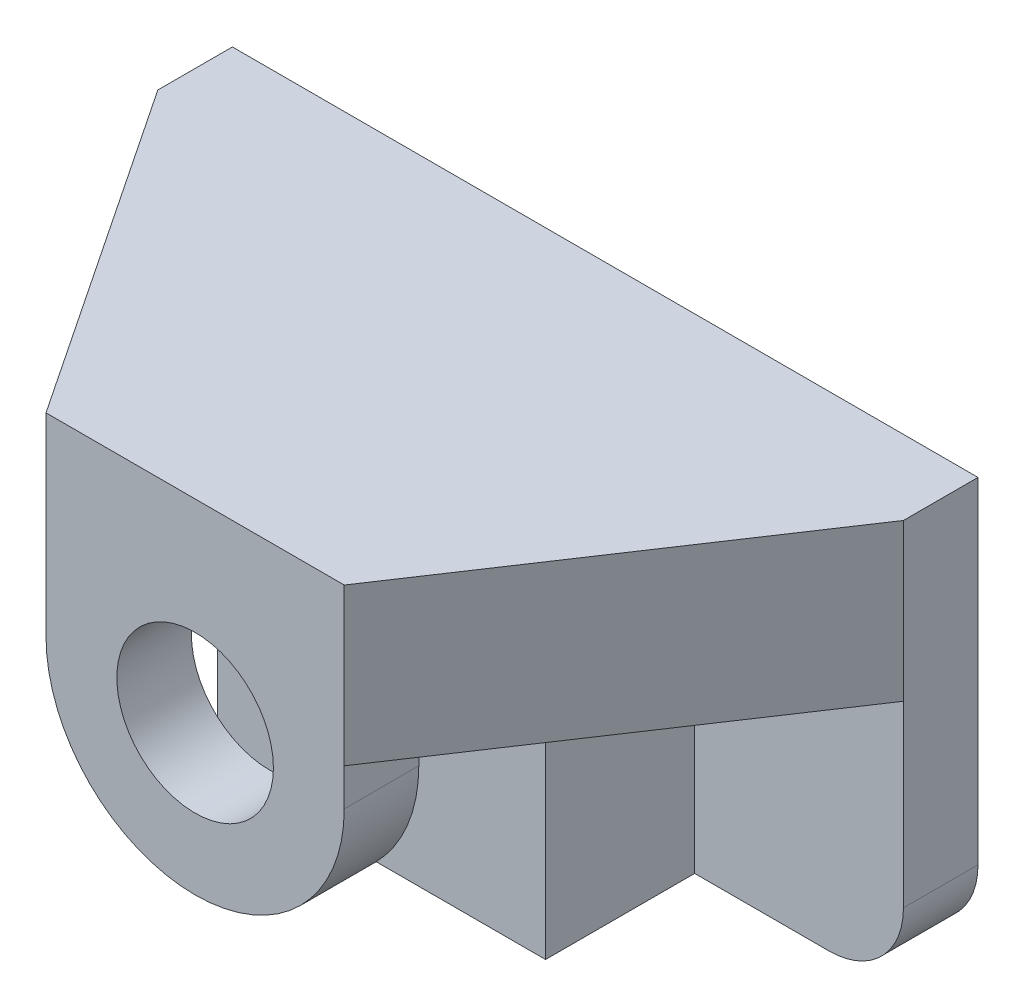
ISO-10303-21;
HEADER;
FILE_DESCRIPTION(('STEP AP214'),'2;1');
FILE_NAME('part.step','',(''),(''),'','','');
FILE_SCHEMA(('AUTOMOTIVE_DESIGN { 1 0 10303 214 1 1 1 1 }'));
ENDSEC;
DATA;
#1=APPLICATION_CONTEXT('core data for automotive mechanical design processes');
#2=APPLICATION_PROTOCOL_DEFINITION('international standard','automotive_design',2000,#1);
#3=PRODUCT_CONTEXT('',#1,'mechanical');
#4=PRODUCT('Part','Part','',(#3));
#5=PRODUCT_RELATED_PRODUCT_CATEGORY('part','',(#4));
#6=PRODUCT_DEFINITION_FORMATION('','',#4);
#7=PRODUCT_DEFINITION_CONTEXT('part definition',#1,'design');
#8=PRODUCT_DEFINITION('design','',#6,#7);
#9=PRODUCT_DEFINITION_SHAPE('','',#8);
#10=(LENGTH_UNIT() NAMED_UNIT(*) SI_UNIT(.MILLI.,.METRE.));
#11=(NAMED_UNIT(*) PLANE_ANGLE_UNIT() SI_UNIT($,.RADIAN.));
#12=(NAMED_UNIT(*) SI_UNIT($,.STERADIAN.) SOLID_ANGLE_UNIT());
#13=UNCERTAINTY_MEASURE_WITH_UNIT(LENGTH_MEASURE(1.E-05),#10,'distance_accuracy_value','');
#14=(GEOMETRIC_REPRESENTATION_CONTEXT(3) GLOBAL_UNCERTAINTY_ASSIGNED_CONTEXT((#13)) GLOBAL_UNIT_ASSIGNED_CONTEXT((#10,
#11,#12)) REPRESENTATION_CONTEXT('',''));
#15=CARTESIAN_POINT('',(0.,0.,0.));
#16=DIRECTION('',(0.,0.,1.));
#17=DIRECTION('',(1.,0.,0.));
#18=AXIS2_PLACEMENT_3D('',#15,#16,#17);
#19=CARTESIAN_POINT('',(0.,-21.,0.));
#20=DIRECTION('',(0.,-1.,0.));
#21=DIRECTION('',(0.,0.,-1.));
#22=AXIS2_PLACEMENT_3D('',#19,#20,#21);
#23=PLANE('',#22);
#24=DIRECTION('',(1.,0.,0.));
#25=VECTOR('',#24,1.);
#26=CARTESIAN_POINT('',(20.,-21.,45.));
#27=LINE('',#26,#25);
#28=CARTESIAN_POINT('',(-20.,-21.,45.));
#29=VERTEX_POINT('',#28);
#30=CARTESIAN_POINT('',(-9.23309265630969,-21.,45.));
#31=VERTEX_POINT('',#30);
#32=EDGE_CURVE('E188',#29,#31,#27,.T.);
#33=ORIENTED_EDGE('',*,*,#32,.F.);
#34=DIRECTION('',(0.,0.,-1.));
#35=VECTOR('',#34,1.);
#36=CARTESIAN_POINT('',(-20.,-21.,45.));
#37=LINE('',#36,#35);
#38=CARTESIAN_POINT('',(-20.,-21.,55.));
#39=VERTEX_POINT('',#38);
#40=EDGE_CURVE('E205',#39,#29,#37,.T.);
#41=ORIENTED_EDGE('',*,*,#40,.F.);
#42=DIRECTION('',(0.554700196225229,0.,0.832050294337844));
#43=VECTOR('',#42,1.);
#44=CARTESIAN_POINT('',(-20.,-21.,55.));
#45=LINE('',#44,#43);
#46=CARTESIAN_POINT('',(-50.,-21.,10.));
#47=VERTEX_POINT('',#46);
#48=EDGE_CURVE('E247',#47,#39,#45,.T.);
#49=ORIENTED_EDGE('',*,*,#48,.F.);
#50=DIRECTION('',(-1.,0.,0.));
#51=VECTOR('',#50,1.);
#52=CARTESIAN_POINT('',(50.,-21.,10.));
#53=LINE('',#52,#51);
#54=CARTESIAN_POINT('',(-22.,-21.,10.));
#55=VERTEX_POINT('',#54);
#56=EDGE_CURVE('E259',#55,#47,#53,.T.);
#57=ORIENTED_EDGE('',*,*,#56,.F.);
#58=DIRECTION('',(0.,0.,1.));
#59=VECTOR('',#58,1.);
#60=CARTESIAN_POINT('',(-22.,-21.,30.));
#61=LINE('',#60,#59);
#62=CARTESIAN_POINT('',(-22.,-21.,30.));
#63=VERTEX_POINT('',#62);
#64=EDGE_CURVE('E267',#55,#63,#61,.T.);
#65=ORIENTED_EDGE('',*,*,#64,.T.);
#66=DIRECTION('',(1.,0.,0.));
#67=VECTOR('',#66,1.);
#68=CARTESIAN_POINT('',(22.0000000000001,-21.,30.));
#69=LINE('',#68,#67);
#70=CARTESIAN_POINT('',(22.0000000000001,-21.,30.));
#71=VERTEX_POINT('',#70);
#72=EDGE_CURVE('E273',#63,#71,#69,.T.);
#73=ORIENTED_EDGE('',*,*,#72,.T.);
#74=DIRECTION('',(0.,0.,-1.));
#75=VECTOR('',#74,1.);
#76=CARTESIAN_POINT('',(22.0000000000001,-21.,10.));
#77=LINE('',#76,#75);
#78=CARTESIAN_POINT('',(22.0000000000001,-21.,10.));
#79=VERTEX_POINT('',#78);
#80=EDGE_CURVE('E279',#71,#79,#77,.T.);
#81=ORIENTED_EDGE('',*,*,#80,.T.);
#82=CARTESIAN_POINT('',(50.,-21.,10.));
#83=VERTEX_POINT('',#82);
#84=EDGE_CURVE('E371',#83,#79,#53,.T.);
#85=ORIENTED_EDGE('',*,*,#84,.F.);
#86=DIRECTION('',(0.554700196225229,0.,-0.832050294337844));
#87=VECTOR('',#86,1.);
#88=CARTESIAN_POINT('',(20.,-21.,55.));
#89=LINE('',#88,#87);
#90=CARTESIAN_POINT('',(20.,-21.,55.));
#91=VERTEX_POINT('',#90);
#92=EDGE_CURVE('E253',#91,#83,#89,.T.);
#93=ORIENTED_EDGE('',*,*,#92,.F.);
#94=DIRECTION('',(0.,0.,1.));
#95=VECTOR('',#94,1.);
#96=CARTESIAN_POINT('',(20.,-21.,55.));
#97=LINE('',#96,#95);
#98=CARTESIAN_POINT('',(20.,-21.,45.));
#99=VERTEX_POINT('',#98);
#100=EDGE_CURVE('E196',#99,#91,#97,.T.);
#101=ORIENTED_EDGE('',*,*,#100,.F.);
#102=CARTESIAN_POINT('',(9.23309265630969,-21.,45.));
#103=VERTEX_POINT('',#102);
#104=EDGE_CURVE('E195',#103,#99,#27,.T.);
#105=ORIENTED_EDGE('',*,*,#104,.F.);
#106=EDGE_CURVE('E182',#31,#103,#27,.T.);
#107=ORIENTED_EDGE('',*,*,#106,.F.);
#108=EDGE_LOOP('',(#33,#41,#49,#57,#65,#73,#81,#85,#93,#101,#105,#107));
#109=FACE_BOUND('',#108,.T.);
#110=ADVANCED_FACE('F50',(#109),#23,.T.);
#111=CARTESIAN_POINT('',(0.,0.,10.));
#112=DIRECTION('',(0.,0.,1.));
#113=DIRECTION('',(1.,0.,0.));
#114=AXIS2_PLACEMENT_3D('',#111,#112,#113);
#115=PLANE('',#114);
#116=ORIENTED_EDGE('',*,*,#56,.T.);
#117=DIRECTION('',(0.,-1.,0.));
#118=VECTOR('',#117,1.);
#119=CARTESIAN_POINT('',(-50.,0.,10.));
#120=LINE('',#119,#118);
#121=CARTESIAN_POINT('',(-50.,-45.,10.));
#122=VERTEX_POINT('',#121);
#123=EDGE_CURVE('E303',#47,#122,#120,.T.);
#124=ORIENTED_EDGE('',*,*,#123,.T.);
#125=CARTESIAN_POINT('',(-40.,-45.,10.));
#126=DIRECTION('',(0.,0.,1.));
#127=DIRECTION('',(1.,0.,0.));
#128=AXIS2_PLACEMENT_3D('',#125,#126,#127);
#129=CIRCLE('',#128,9.99999999999999);
#130=CARTESIAN_POINT('',(-40.,-55.,10.));
#131=VERTEX_POINT('',#130);
#132=EDGE_CURVE('E306',#122,#131,#129,.T.);
#133=ORIENTED_EDGE('',*,*,#132,.T.);
#134=DIRECTION('',(1.,0.,0.));
#135=VECTOR('',#134,1.);
#136=CARTESIAN_POINT('',(0.,-55.,10.));
#137=LINE('',#136,#135);
#138=CARTESIAN_POINT('',(-22.,-55.,10.));
#139=VERTEX_POINT('',#138);
#140=EDGE_CURVE('E308',#131,#139,#137,.T.);
#141=ORIENTED_EDGE('',*,*,#140,.T.);
#142=DIRECTION('',(0.,1.,0.));
#143=VECTOR('',#142,1.);
#144=CARTESIAN_POINT('',(-22.,0.,10.));
#145=LINE('',#144,#143);
#146=EDGE_CURVE('E311',#139,#55,#145,.T.);
#147=ORIENTED_EDGE('',*,*,#146,.T.);
#148=EDGE_LOOP('',(#116,#124,#133,#141,#147));
#149=FACE_BOUND('',#148,.T.);
#150=ADVANCED_FACE('F415',(#149),#115,.T.);
#151=ORIENTED_EDGE('',*,*,#84,.T.);
#152=DIRECTION('',(0.,1.,0.));
#153=VECTOR('',#152,1.);
#154=CARTESIAN_POINT('',(22.0000000000001,0.,10.));
#155=LINE('',#154,#153);
#156=CARTESIAN_POINT('',(22.0000000000001,-55.,10.));
#157=VERTEX_POINT('',#156);
#158=EDGE_CURVE('E312',#157,#79,#155,.T.);
#159=ORIENTED_EDGE('',*,*,#158,.F.);
#160=DIRECTION('',(-1.,0.,0.));
#161=VECTOR('',#160,1.);
#162=CARTESIAN_POINT('',(0.,-55.,10.));
#163=LINE('',#162,#161);
#164=CARTESIAN_POINT('',(40.0000000000001,-55.,10.));
#165=VERTEX_POINT('',#164);
#166=EDGE_CURVE('E294',#165,#157,#163,.T.);
#167=ORIENTED_EDGE('',*,*,#166,.F.);
#168=CARTESIAN_POINT('',(40.,-45.,10.));
#169=DIRECTION('',(0.,0.,1.));
#170=DIRECTION('',(1.,0.,0.));
#171=AXIS2_PLACEMENT_3D('',#168,#169,#170);
#172=CIRCLE('',#171,10.);
#173=CARTESIAN_POINT('',(50.,-45.,10.));
#174=VERTEX_POINT('',#173);
#175=EDGE_CURVE('E296',#165,#174,#172,.T.);
#176=ORIENTED_EDGE('',*,*,#175,.T.);
#177=DIRECTION('',(0.,-1.,0.));
#178=VECTOR('',#177,1.);
#179=CARTESIAN_POINT('',(50.,0.,10.));
#180=LINE('',#179,#178);
#181=EDGE_CURVE('E69',#83,#174,#180,.T.);
#182=ORIENTED_EDGE('',*,*,#181,.F.);
#183=EDGE_LOOP('',(#151,#159,#167,#176,#182));
#184=FACE_BOUND('',#183,.T.);
#185=ADVANCED_FACE('F395',(#184),#115,.T.);
#186=CARTESIAN_POINT('',(40.,-45.,10.));
#187=DIRECTION('',(0.,0.,-1.));
#188=DIRECTION('',(-1.,0.,0.));
#189=AXIS2_PLACEMENT_3D('',#186,#187,#188);
#190=CYLINDRICAL_SURFACE('',#189,10.);
#191=CARTESIAN_POINT('',(40.,-45.,0.));
#192=DIRECTION('',(0.,0.,1.));
#193=DIRECTION('',(1.,0.,0.));
#194=AXIS2_PLACEMENT_3D('',#191,#192,#193);
#195=CIRCLE('',#194,10.);
#196=CARTESIAN_POINT('',(40.0000000000001,-55.,0.));
#197=VERTEX_POINT('',#196);
#198=CARTESIAN_POINT('',(50.,-45.,0.));
#199=VERTEX_POINT('',#198);
#200=EDGE_CURVE('E295',#197,#199,#195,.T.);
#201=ORIENTED_EDGE('',*,*,#200,.T.);
#202=DIRECTION('',(0.,0.,-1.));
#203=VECTOR('',#202,1.);
#204=CARTESIAN_POINT('',(50.,-45.,10.));
#205=LINE('',#204,#203);
#206=EDGE_CURVE('E338',#174,#199,#205,.T.);
#207=ORIENTED_EDGE('',*,*,#206,.F.);
#208=ORIENTED_EDGE('',*,*,#175,.F.);
#209=DIRECTION('',(0.,0.,-1.));
#210=VECTOR('',#209,1.);
#211=CARTESIAN_POINT('',(40.0000000000001,-55.,10.));
#212=LINE('',#211,#210);
#213=EDGE_CURVE('E345',#165,#197,#212,.T.);
#214=ORIENTED_EDGE('',*,*,#213,.T.);
#215=EDGE_LOOP('',(#201,#207,#208,#214));
#216=FACE_BOUND('',#215,.T.);
#217=ADVANCED_FACE('F47',(#216),#190,.T.);
#218=CARTESIAN_POINT('',(50.,0.,10.));
#219=DIRECTION('',(1.,0.,0.));
#220=DIRECTION('',(0.,0.,-1.));
#221=AXIS2_PLACEMENT_3D('',#218,#219,#220);
#222=PLANE('',#221);
#223=DIRECTION('',(0.,-1.,0.));
#224=VECTOR('',#223,1.);
#225=CARTESIAN_POINT('',(50.,0.,0.));
#226=LINE('',#225,#224);
#227=CARTESIAN_POINT('',(50.,0.,0.));
#228=VERTEX_POINT('',#227);
#229=EDGE_CURVE('E316',#228,#199,#226,.T.);
#230=ORIENTED_EDGE('',*,*,#229,.F.);
#231=DIRECTION('',(0.,0.,-1.));
#232=VECTOR('',#231,1.);
#233=CARTESIAN_POINT('',(50.,0.,10.));
#234=LINE('',#233,#232);
#235=CARTESIAN_POINT('',(50.,0.,10.));
#236=VERTEX_POINT('',#235);
#237=EDGE_CURVE('E336',#236,#228,#234,.T.);
#238=ORIENTED_EDGE('',*,*,#237,.F.);
#239=EDGE_CURVE('E301',#236,#83,#180,.T.);
#240=ORIENTED_EDGE('',*,*,#239,.T.);
#241=ORIENTED_EDGE('',*,*,#181,.T.);
#242=ORIENTED_EDGE('',*,*,#206,.T.);
#243=EDGE_LOOP('',(#230,#238,#240,#241,#242));
#244=FACE_BOUND('',#243,.T.);
#245=ADVANCED_FACE('F401',(#244),#222,.T.);
#246=CARTESIAN_POINT('',(0.,0.,10.));
#247=DIRECTION('',(0.,1.,0.));
#248=DIRECTION('',(0.,0.,1.));
#249=AXIS2_PLACEMENT_3D('',#246,#247,#248);
#250=PLANE('',#249);
#251=DIRECTION('',(1.,0.,0.));
#252=VECTOR('',#251,1.);
#253=CARTESIAN_POINT('',(0.,0.,0.));
#254=LINE('',#253,#252);
#255=CARTESIAN_POINT('',(-50.,0.,0.));
#256=VERTEX_POINT('',#255);
#257=EDGE_CURVE('E325',#256,#228,#254,.T.);
#258=ORIENTED_EDGE('',*,*,#257,.F.);
#259=DIRECTION('',(0.,0.,-1.));
#260=VECTOR('',#259,1.);
#261=CARTESIAN_POINT('',(-50.,0.,10.));
#262=LINE('',#261,#260);
#263=CARTESIAN_POINT('',(-50.,0.,10.));
#264=VERTEX_POINT('',#263);
#265=EDGE_CURVE('E254',#264,#256,#262,.T.);
#266=ORIENTED_EDGE('',*,*,#265,.F.);
#267=DIRECTION('',(0.554700196225229,0.,0.832050294337844));
#268=VECTOR('',#267,1.);
#269=CARTESIAN_POINT('',(-20.,0.,55.));
#270=LINE('',#269,#268);
#271=CARTESIAN_POINT('',(-20.,0.,55.));
#272=VERTEX_POINT('',#271);
#273=EDGE_CURVE('E246',#264,#272,#270,.T.);
#274=ORIENTED_EDGE('',*,*,#273,.T.);
#275=DIRECTION('',(1.,0.,0.));
#276=VECTOR('',#275,1.);
#277=CARTESIAN_POINT('',(0.,0.,55.));
#278=LINE('',#277,#276);
#279=CARTESIAN_POINT('',(20.,0.,55.));
#280=VERTEX_POINT('',#279);
#281=EDGE_CURVE('E230',#272,#280,#278,.T.);
#282=ORIENTED_EDGE('',*,*,#281,.T.);
#283=DIRECTION('',(0.554700196225229,0.,-0.832050294337844));
#284=VECTOR('',#283,1.);
#285=CARTESIAN_POINT('',(20.,0.,55.));
#286=LINE('',#285,#284);
#287=EDGE_CURVE('E239',#280,#236,#286,.T.);
#288=ORIENTED_EDGE('',*,*,#287,.T.);
#289=ORIENTED_EDGE('',*,*,#237,.T.);
#290=EDGE_LOOP('',(#258,#266,#274,#282,#288,#289));
#291=FACE_BOUND('',#290,.T.);
#292=ADVANCED_FACE('F255',(#291),#250,.T.);
#293=CARTESIAN_POINT('',(-50.,0.,10.));
#294=DIRECTION('',(1.,0.,0.));
#295=DIRECTION('',(0.,0.,-1.));
#296=AXIS2_PLACEMENT_3D('',#293,#294,#295);
#297=PLANE('',#296);
#298=DIRECTION('',(0.,-1.,0.));
#299=VECTOR('',#298,1.);
#300=CARTESIAN_POINT('',(-50.,0.,0.));
#301=LINE('',#300,#299);
#302=CARTESIAN_POINT('',(-50.,-45.,0.));
#303=VERTEX_POINT('',#302);
#304=EDGE_CURVE('E323',#256,#303,#301,.T.);
#305=ORIENTED_EDGE('',*,*,#304,.T.);
#306=DIRECTION('',(0.,0.,-1.));
#307=VECTOR('',#306,1.);
#308=CARTESIAN_POINT('',(-50.,-45.,10.));
#309=LINE('',#308,#307);
#310=EDGE_CURVE('E333',#122,#303,#309,.T.);
#311=ORIENTED_EDGE('',*,*,#310,.F.);
#312=ORIENTED_EDGE('',*,*,#123,.F.);
#313=EDGE_CURVE('E302',#264,#47,#120,.T.);
#314=ORIENTED_EDGE('',*,*,#313,.F.);
#315=ORIENTED_EDGE('',*,*,#265,.T.);
#316=EDGE_LOOP('',(#305,#311,#312,#314,#315));
#317=FACE_BOUND('',#316,.T.);
#318=ADVANCED_FACE('F367',(#317),#297,.F.);
#319=CARTESIAN_POINT('',(-40.,-45.,10.));
#320=DIRECTION('',(0.,0.,-1.));
#321=DIRECTION('',(-1.,0.,0.));
#322=AXIS2_PLACEMENT_3D('',#319,#320,#321);
#323=CYLINDRICAL_SURFACE('',#322,9.99999999999999);
#324=CARTESIAN_POINT('',(-40.,-45.,0.));
#325=DIRECTION('',(0.,0.,1.));
#326=DIRECTION('',(1.,0.,0.));
#327=AXIS2_PLACEMENT_3D('',#324,#325,#326);
#328=CIRCLE('',#327,9.99999999999999);
#329=CARTESIAN_POINT('',(-40.,-55.,0.));
#330=VERTEX_POINT('',#329);
#331=EDGE_CURVE('E330',#303,#330,#328,.T.);
#332=ORIENTED_EDGE('',*,*,#331,.T.);
#333=DIRECTION('',(0.,0.,-1.));
#334=VECTOR('',#333,1.);
#335=CARTESIAN_POINT('',(-40.,-55.,10.));
#336=LINE('',#335,#334);
#337=EDGE_CURVE('E317',#131,#330,#336,.T.);
#338=ORIENTED_EDGE('',*,*,#337,.F.);
#339=ORIENTED_EDGE('',*,*,#132,.F.);
#340=ORIENTED_EDGE('',*,*,#310,.T.);
#341=EDGE_LOOP('',(#332,#338,#339,#340));
#342=FACE_BOUND('',#341,.T.);
#343=ADVANCED_FACE('F364',(#342),#323,.T.);
#344=CARTESIAN_POINT('',(0.,-55.,10.));
#345=DIRECTION('',(0.,1.,0.));
#346=DIRECTION('',(0.,0.,1.));
#347=AXIS2_PLACEMENT_3D('',#344,#345,#346);
#348=PLANE('',#347);
#349=DIRECTION('',(1.,0.,0.));
#350=VECTOR('',#349,1.);
#351=CARTESIAN_POINT('',(0.,-55.,0.));
#352=LINE('',#351,#350);
#353=CARTESIAN_POINT('',(-19.9999999999999,-55.,0.));
#354=VERTEX_POINT('',#353);
#355=EDGE_CURVE('E299',#330,#354,#352,.T.);
#356=ORIENTED_EDGE('',*,*,#355,.T.);
#357=CARTESIAN_POINT('',(0.,-55.,0.));
#358=DIRECTION('',(0.,-1.,0.));
#359=DIRECTION('',(0.,0.,-1.));
#360=AXIS2_PLACEMENT_3D('',#357,#358,#359);
#361=CIRCLE('',#360,20.);
#362=CARTESIAN_POINT('',(20.0000000000001,-55.,0.));
#363=VERTEX_POINT('',#362);
#364=EDGE_CURVE('E248',#363,#354,#361,.T.);
#365=ORIENTED_EDGE('',*,*,#364,.F.);
#366=EDGE_CURVE('E329',#363,#197,#352,.T.);
#367=ORIENTED_EDGE('',*,*,#366,.T.);
#368=ORIENTED_EDGE('',*,*,#213,.F.);
#369=ORIENTED_EDGE('',*,*,#166,.T.);
#370=DIRECTION('',(0.,0.,1.));
#371=VECTOR('',#370,1.);
#372=CARTESIAN_POINT('',(22.0000000000001,-55.,0.));
#373=LINE('',#372,#371);
#374=CARTESIAN_POINT('',(22.0000000000001,-55.,30.));
#375=VERTEX_POINT('',#374);
#376=EDGE_CURVE('E284',#157,#375,#373,.T.);
#377=ORIENTED_EDGE('',*,*,#376,.T.);
#378=DIRECTION('',(-1.,0.,0.));
#379=VECTOR('',#378,1.);
#380=CARTESIAN_POINT('',(22.0000000000001,-55.,30.));
#381=LINE('',#380,#379);
#382=CARTESIAN_POINT('',(-22.,-55.,30.));
#383=VERTEX_POINT('',#382);
#384=EDGE_CURVE('E289',#375,#383,#381,.T.);
#385=ORIENTED_EDGE('',*,*,#384,.T.);
#386=DIRECTION('',(0.,0.,-1.));
#387=VECTOR('',#386,1.);
#388=CARTESIAN_POINT('',(-22.,-55.,10.));
#389=LINE('',#388,#387);
#390=EDGE_CURVE('E283',#383,#139,#389,.T.);
#391=ORIENTED_EDGE('',*,*,#390,.T.);
#392=ORIENTED_EDGE('',*,*,#140,.F.);
#393=ORIENTED_EDGE('',*,*,#337,.T.);
#394=EDGE_LOOP('',(#356,#365,#367,#368,#369,#377,#385,#391,#392,#393));
#395=FACE_BOUND('',#394,.T.);
#396=ADVANCED_FACE('F356',(#395),#348,.F.);
#397=CARTESIAN_POINT('',(0.,0.,0.));
#398=DIRECTION('',(0.,0.,1.));
#399=DIRECTION('',(1.,0.,0.));
#400=AXIS2_PLACEMENT_3D('',#397,#398,#399);
#401=PLANE('',#400);
#402=DIRECTION('',(1.,0.,0.));
#403=VECTOR('',#402,1.);
#404=CARTESIAN_POINT('',(-19.9999999999999,-21.,0.));
#405=LINE('',#404,#403);
#406=CARTESIAN_POINT('',(-19.9999999999999,-21.,0.));
#407=VERTEX_POINT('',#406);
#408=CARTESIAN_POINT('',(20.0000000000001,-21.,0.));
#409=VERTEX_POINT('',#408);
#410=EDGE_CURVE('E261',#407,#409,#405,.T.);
#411=ORIENTED_EDGE('',*,*,#410,.F.);
#412=DIRECTION('',(0.,-1.,0.));
#413=VECTOR('',#412,1.);
#414=CARTESIAN_POINT('',(-19.9999999999999,-21.,0.));
#415=LINE('',#414,#413);
#416=EDGE_CURVE('E269',#407,#354,#415,.T.);
#417=ORIENTED_EDGE('',*,*,#416,.T.);
#418=ORIENTED_EDGE('',*,*,#355,.F.);
#419=ORIENTED_EDGE('',*,*,#331,.F.);
#420=ORIENTED_EDGE('',*,*,#304,.F.);
#421=ORIENTED_EDGE('',*,*,#257,.T.);
#422=ORIENTED_EDGE('',*,*,#229,.T.);
#423=ORIENTED_EDGE('',*,*,#200,.F.);
#424=ORIENTED_EDGE('',*,*,#366,.F.);
#425=DIRECTION('',(0.,-1.,0.));
#426=VECTOR('',#425,1.);
#427=CARTESIAN_POINT('',(20.0000000000001,-21.,0.));
#428=LINE('',#427,#426);
#429=EDGE_CURVE('E270',#409,#363,#428,.T.);
#430=ORIENTED_EDGE('',*,*,#429,.F.);
#431=EDGE_LOOP('',(#411,#417,#418,#419,#420,#421,#422,#423,#424,#430));
#432=FACE_BOUND('',#431,.T.);
#433=ADVANCED_FACE('F353',(#432),#401,.F.);
#434=CARTESIAN_POINT('',(22.0000000000001,-55.,10.));
#435=DIRECTION('',(-1.,0.,0.));
#436=DIRECTION('',(0.,0.,1.));
#437=AXIS2_PLACEMENT_3D('',#434,#435,#436);
#438=PLANE('',#437);
#439=ORIENTED_EDGE('',*,*,#158,.T.);
#440=ORIENTED_EDGE('',*,*,#80,.F.);
#441=DIRECTION('',(0.,1.,0.));
#442=VECTOR('',#441,1.);
#443=CARTESIAN_POINT('',(22.0000000000001,-55.,30.));
#444=LINE('',#443,#442);
#445=EDGE_CURVE('E292',#375,#71,#444,.T.);
#446=ORIENTED_EDGE('',*,*,#445,.F.);
#447=ORIENTED_EDGE('',*,*,#376,.F.);
#448=EDGE_LOOP('',(#439,#440,#446,#447));
#449=FACE_BOUND('',#448,.T.);
#450=ADVANCED_FACE('F392',(#449),#438,.F.);
#451=CARTESIAN_POINT('',(22.0000000000001,-55.,30.));
#452=DIRECTION('',(0.,0.,-1.));
#453=DIRECTION('',(-1.,0.,0.));
#454=AXIS2_PLACEMENT_3D('',#451,#452,#453);
#455=PLANE('',#454);
#456=ORIENTED_EDGE('',*,*,#445,.T.);
#457=ORIENTED_EDGE('',*,*,#72,.F.);
#458=DIRECTION('',(0.,1.,0.));
#459=VECTOR('',#458,1.);
#460=CARTESIAN_POINT('',(-22.,-55.,30.));
#461=LINE('',#460,#459);
#462=EDGE_CURVE('E288',#383,#63,#461,.T.);
#463=ORIENTED_EDGE('',*,*,#462,.F.);
#464=ORIENTED_EDGE('',*,*,#384,.F.);
#465=EDGE_LOOP('',(#456,#457,#463,#464));
#466=FACE_BOUND('',#465,.T.);
#467=ADVANCED_FACE('F433',(#466),#455,.F.);
#468=CARTESIAN_POINT('',(-22.,-55.,10.));
#469=DIRECTION('',(1.,0.,0.));
#470=DIRECTION('',(0.,0.,-1.));
#471=AXIS2_PLACEMENT_3D('',#468,#469,#470);
#472=PLANE('',#471);
#473=ORIENTED_EDGE('',*,*,#146,.F.);
#474=ORIENTED_EDGE('',*,*,#390,.F.);
#475=ORIENTED_EDGE('',*,*,#462,.T.);
#476=ORIENTED_EDGE('',*,*,#64,.F.);
#477=EDGE_LOOP('',(#473,#474,#475,#476));
#478=FACE_BOUND('',#477,.T.);
#479=ADVANCED_FACE('F427',(#478),#472,.F.);
#480=CARTESIAN_POINT('',(0.,-21.,0.));
#481=DIRECTION('',(0.,-1.,0.));
#482=DIRECTION('',(0.,0.,-1.));
#483=AXIS2_PLACEMENT_3D('',#480,#481,#482);
#484=CYLINDRICAL_SURFACE('',#483,20.);
#485=ORIENTED_EDGE('',*,*,#364,.T.);
#486=ORIENTED_EDGE('',*,*,#416,.F.);
#487=CARTESIAN_POINT('',(0.,-21.,0.));
#488=DIRECTION('',(0.,-1.,0.));
#489=DIRECTION('',(0.,0.,-1.));
#490=AXIS2_PLACEMENT_3D('',#487,#488,#489);
#491=CIRCLE('',#490,20.);
#492=EDGE_CURVE('E54',#409,#407,#491,.T.);
#493=ORIENTED_EDGE('',*,*,#492,.F.);
#494=ORIENTED_EDGE('',*,*,#429,.T.);
#495=EDGE_LOOP('',(#485,#486,#493,#494));
#496=FACE_BOUND('',#495,.T.);
#497=ADVANCED_FACE('F347',(#496),#484,.F.);
#498=CARTESIAN_POINT('',(0.,-21.,0.));
#499=DIRECTION('',(0.,-1.,0.));
#500=DIRECTION('',(0.,0.,-1.));
#501=AXIS2_PLACEMENT_3D('',#498,#499,#500);
#502=PLANE('',#501);
#503=ORIENTED_EDGE('',*,*,#492,.T.);
#504=ORIENTED_EDGE('',*,*,#410,.T.);
#505=EDGE_LOOP('',(#503,#504));
#506=FACE_BOUND('',#505,.T.);
#507=ADVANCED_FACE('F348',(#506),#502,.T.);
#508=CARTESIAN_POINT('',(-20.,-21.,55.));
#509=DIRECTION('',(-0.832050294337843,0.,0.554700196225229));
#510=DIRECTION('',(0.554700196225229,0.,0.832050294337844));
#511=AXIS2_PLACEMENT_3D('',#508,#509,#510);
#512=PLANE('',#511);
#513=ORIENTED_EDGE('',*,*,#273,.F.);
#514=ORIENTED_EDGE('',*,*,#313,.T.);
#515=ORIENTED_EDGE('',*,*,#48,.T.);
#516=DIRECTION('',(0.,1.,0.));
#517=VECTOR('',#516,1.);
#518=CARTESIAN_POINT('',(-20.,-21.,55.));
#519=LINE('',#518,#517);
#520=EDGE_CURVE('E235',#39,#272,#519,.T.);
#521=ORIENTED_EDGE('',*,*,#520,.T.);
#522=EDGE_LOOP('',(#513,#514,#515,#521));
#523=FACE_BOUND('',#522,.T.);
#524=ADVANCED_FACE('F242',(#523),#512,.T.);
#525=CARTESIAN_POINT('',(20.,-21.,55.));
#526=DIRECTION('',(0.832050294337843,0.,0.554700196225229));
#527=DIRECTION('',(0.554700196225229,0.,-0.832050294337844));
#528=AXIS2_PLACEMENT_3D('',#525,#526,#527);
#529=PLANE('',#528);
#530=ORIENTED_EDGE('',*,*,#287,.F.);
#531=DIRECTION('',(0.,1.,0.));
#532=VECTOR('',#531,1.);
#533=CARTESIAN_POINT('',(20.,-21.,55.));
#534=LINE('',#533,#532);
#535=EDGE_CURVE('E232',#91,#280,#534,.T.);
#536=ORIENTED_EDGE('',*,*,#535,.F.);
#537=ORIENTED_EDGE('',*,*,#92,.T.);
#538=ORIENTED_EDGE('',*,*,#239,.F.);
#539=EDGE_LOOP('',(#530,#536,#537,#538));
#540=FACE_BOUND('',#539,.T.);
#541=ADVANCED_FACE('F222',(#540),#529,.T.);
#542=CARTESIAN_POINT('',(0.,-21.,55.));
#543=DIRECTION('',(0.,0.,1.));
#544=DIRECTION('',(1.,0.,0.));
#545=AXIS2_PLACEMENT_3D('',#542,#543,#544);
#546=PLANE('',#545);
#547=CARTESIAN_POINT('',(0.,-26.,55.));
#548=DIRECTION('',(0.,0.,1.));
#549=DIRECTION('',(1.,0.,0.));
#550=AXIS2_PLACEMENT_3D('',#547,#548,#549);
#551=CIRCLE('',#550,10.5);
#552=CARTESIAN_POINT('',(10.5,-26.,55.));
#553=VERTEX_POINT('',#552);
#554=EDGE_CURVE('E184',#553,#553,#551,.T.);
#555=ORIENTED_EDGE('',*,*,#554,.F.);
#556=EDGE_LOOP('',(#555));
#557=FACE_BOUND('',#556,.T.);
#558=ORIENTED_EDGE('',*,*,#281,.F.);
#559=ORIENTED_EDGE('',*,*,#520,.F.);
#560=DIRECTION('',(0.,1.,0.));
#561=VECTOR('',#560,1.);
#562=CARTESIAN_POINT('',(-20.,-26.,55.));
#563=LINE('',#562,#561);
#564=CARTESIAN_POINT('',(-20.,-26.,55.));
#565=VERTEX_POINT('',#564);
#566=EDGE_CURVE('E214',#565,#39,#563,.T.);
#567=ORIENTED_EDGE('',*,*,#566,.F.);
#568=CARTESIAN_POINT('',(0.,-26.,55.));
#569=DIRECTION('',(0.,0.,1.));
#570=DIRECTION('',(1.,0.,0.));
#571=AXIS2_PLACEMENT_3D('',#568,#569,#570);
#572=CIRCLE('',#571,20.);
#573=CARTESIAN_POINT('',(20.,-26.,55.));
#574=VERTEX_POINT('',#573);
#575=EDGE_CURVE('E183',#565,#574,#572,.T.);
#576=ORIENTED_EDGE('',*,*,#575,.T.);
#577=DIRECTION('',(0.,1.,0.));
#578=VECTOR('',#577,1.);
#579=CARTESIAN_POINT('',(20.,-26.,55.));
#580=LINE('',#579,#578);
#581=EDGE_CURVE('E377',#574,#91,#580,.T.);
#582=ORIENTED_EDGE('',*,*,#581,.T.);
#583=ORIENTED_EDGE('',*,*,#535,.T.);
#584=EDGE_LOOP('',(#558,#559,#567,#576,#582,#583));
#585=FACE_BOUND('',#584,.T.);
#586=ADVANCED_FACE('F224',(#557,#585),#546,.T.);
#587=CARTESIAN_POINT('',(-20.,-26.,45.));
#588=DIRECTION('',(1.,0.,0.));
#589=DIRECTION('',(0.,0.,-1.));
#590=AXIS2_PLACEMENT_3D('',#587,#588,#589);
#591=PLANE('',#590);
#592=ORIENTED_EDGE('',*,*,#40,.T.);
#593=DIRECTION('',(0.,1.,0.));
#594=VECTOR('',#593,1.);
#595=CARTESIAN_POINT('',(-20.,-26.,45.));
#596=LINE('',#595,#594);
#597=CARTESIAN_POINT('',(-20.,-26.,45.));
#598=VERTEX_POINT('',#597);
#599=EDGE_CURVE('E198',#598,#29,#596,.T.);
#600=ORIENTED_EDGE('',*,*,#599,.F.);
#601=DIRECTION('',(0.,0.,-1.));
#602=VECTOR('',#601,1.);
#603=CARTESIAN_POINT('',(-20.,-26.,45.));
#604=LINE('',#603,#602);
#605=EDGE_CURVE('E197',#565,#598,#604,.T.);
#606=ORIENTED_EDGE('',*,*,#605,.F.);
#607=ORIENTED_EDGE('',*,*,#566,.T.);
#608=EDGE_LOOP('',(#592,#600,#606,#607));
#609=FACE_BOUND('',#608,.T.);
#610=ADVANCED_FACE('F223',(#609),#591,.F.);
#611=CARTESIAN_POINT('',(20.,-26.,45.));
#612=DIRECTION('',(0.,0.,1.));
#613=DIRECTION('',(1.,0.,0.));
#614=AXIS2_PLACEMENT_3D('',#611,#612,#613);
#615=PLANE('',#614);
#616=ORIENTED_EDGE('',*,*,#32,.T.);
#617=CARTESIAN_POINT('',(0.,-26.,45.));
#618=DIRECTION('',(0.,0.,1.));
#619=DIRECTION('',(1.,0.,0.));
#620=AXIS2_PLACEMENT_3D('',#617,#618,#619);
#621=CIRCLE('',#620,10.5);
#622=EDGE_CURVE('E11',#31,#103,#621,.T.);
#623=ORIENTED_EDGE('',*,*,#622,.T.);
#624=ORIENTED_EDGE('',*,*,#104,.T.);
#625=DIRECTION('',(0.,1.,0.));
#626=VECTOR('',#625,1.);
#627=CARTESIAN_POINT('',(20.,-26.,45.));
#628=LINE('',#627,#626);
#629=CARTESIAN_POINT('',(20.,-26.,45.));
#630=VERTEX_POINT('',#629);
#631=EDGE_CURVE('E376',#630,#99,#628,.T.);
#632=ORIENTED_EDGE('',*,*,#631,.F.);
#633=CARTESIAN_POINT('',(0.,-26.,45.));
#634=DIRECTION('',(0.,0.,1.));
#635=DIRECTION('',(1.,0.,0.));
#636=AXIS2_PLACEMENT_3D('',#633,#634,#635);
#637=CIRCLE('',#636,20.);
#638=EDGE_CURVE('E202',#598,#630,#637,.T.);
#639=ORIENTED_EDGE('',*,*,#638,.F.);
#640=ORIENTED_EDGE('',*,*,#599,.T.);
#641=EDGE_LOOP('',(#616,#623,#624,#632,#639,#640));
#642=FACE_BOUND('',#641,.T.);
#643=ADVANCED_FACE('F191',(#642),#615,.F.);
#644=CARTESIAN_POINT('',(20.,-26.,55.));
#645=DIRECTION('',(-1.,0.,0.));
#646=DIRECTION('',(0.,0.,1.));
#647=AXIS2_PLACEMENT_3D('',#644,#645,#646);
#648=PLANE('',#647);
#649=ORIENTED_EDGE('',*,*,#100,.T.);
#650=ORIENTED_EDGE('',*,*,#581,.F.);
#651=DIRECTION('',(0.,0.,1.));
#652=VECTOR('',#651,1.);
#653=CARTESIAN_POINT('',(20.,-26.,55.));
#654=LINE('',#653,#652);
#655=EDGE_CURVE('E208',#630,#574,#654,.T.);
#656=ORIENTED_EDGE('',*,*,#655,.F.);
#657=ORIENTED_EDGE('',*,*,#631,.T.);
#658=EDGE_LOOP('',(#649,#650,#656,#657));
#659=FACE_BOUND('',#658,.T.);
#660=ADVANCED_FACE('F383',(#659),#648,.F.);
#661=CARTESIAN_POINT('',(0.,-26.,45.));
#662=DIRECTION('',(0.,0.,1.));
#663=DIRECTION('',(1.,0.,0.));
#664=AXIS2_PLACEMENT_3D('',#661,#662,#663);
#665=CYLINDRICAL_SURFACE('',#664,20.);
#666=ORIENTED_EDGE('',*,*,#575,.F.);
#667=ORIENTED_EDGE('',*,*,#605,.T.);
#668=ORIENTED_EDGE('',*,*,#638,.T.);
#669=ORIENTED_EDGE('',*,*,#655,.T.);
#670=EDGE_LOOP('',(#666,#667,#668,#669));
#671=FACE_BOUND('',#670,.T.);
#672=ADVANCED_FACE('F385',(#671),#665,.T.);
#673=CARTESIAN_POINT('',(0.,-26.,45.));
#674=DIRECTION('',(0.,0.,1.));
#675=DIRECTION('',(1.,0.,0.));
#676=AXIS2_PLACEMENT_3D('',#673,#674,#675);
#677=CYLINDRICAL_SURFACE('',#676,10.5);
#678=CARTESIAN_POINT('',(0.,-26.,45.));
#679=DIRECTION('',(0.,0.,1.));
#680=DIRECTION('',(1.,0.,0.));
#681=AXIS2_PLACEMENT_3D('',#678,#679,#680);
#682=CIRCLE('',#681,10.5);
#683=EDGE_CURVE('E62',#103,#31,#682,.T.);
#684=ORIENTED_EDGE('',*,*,#683,.F.);
#685=ORIENTED_EDGE('',*,*,#622,.F.);
#686=EDGE_LOOP('',(#684,#685));
#687=FACE_BOUND('',#686,.T.);
#688=ORIENTED_EDGE('',*,*,#554,.T.);
#689=EDGE_LOOP('',(#688));
#690=FACE_BOUND('',#689,.T.);
#691=ADVANCED_FACE('F174',(#687,#690),#677,.F.);
#692=CARTESIAN_POINT('',(0.,-26.,45.));
#693=DIRECTION('',(0.,0.,1.));
#694=DIRECTION('',(1.,0.,0.));
#695=AXIS2_PLACEMENT_3D('',#692,#693,#694);
#696=PLANE('',#695);
#697=ORIENTED_EDGE('',*,*,#683,.T.);
#698=ORIENTED_EDGE('',*,*,#106,.T.);
#699=EDGE_LOOP('',(#697,#698));
#700=FACE_BOUND('',#699,.T.);
#701=ADVANCED_FACE('F185',(#700),#696,.T.);
#702=CLOSED_SHELL('',(#110,#150,#185,#217,#245,#292,#318,#343,#396,#433,#450,#467,#479,#497,
#507,#524,#541,#586,#610,#643,#660,#672,#691,#701));
#703=MANIFOLD_SOLID_BREP('B2',#702);
#704=ADVANCED_BREP_SHAPE_REPRESENTATION('',(#18,#703),#14);
#705=SHAPE_DEFINITION_REPRESENTATION(#9,#704);
ENDSEC;
END-ISO-10303-21;
